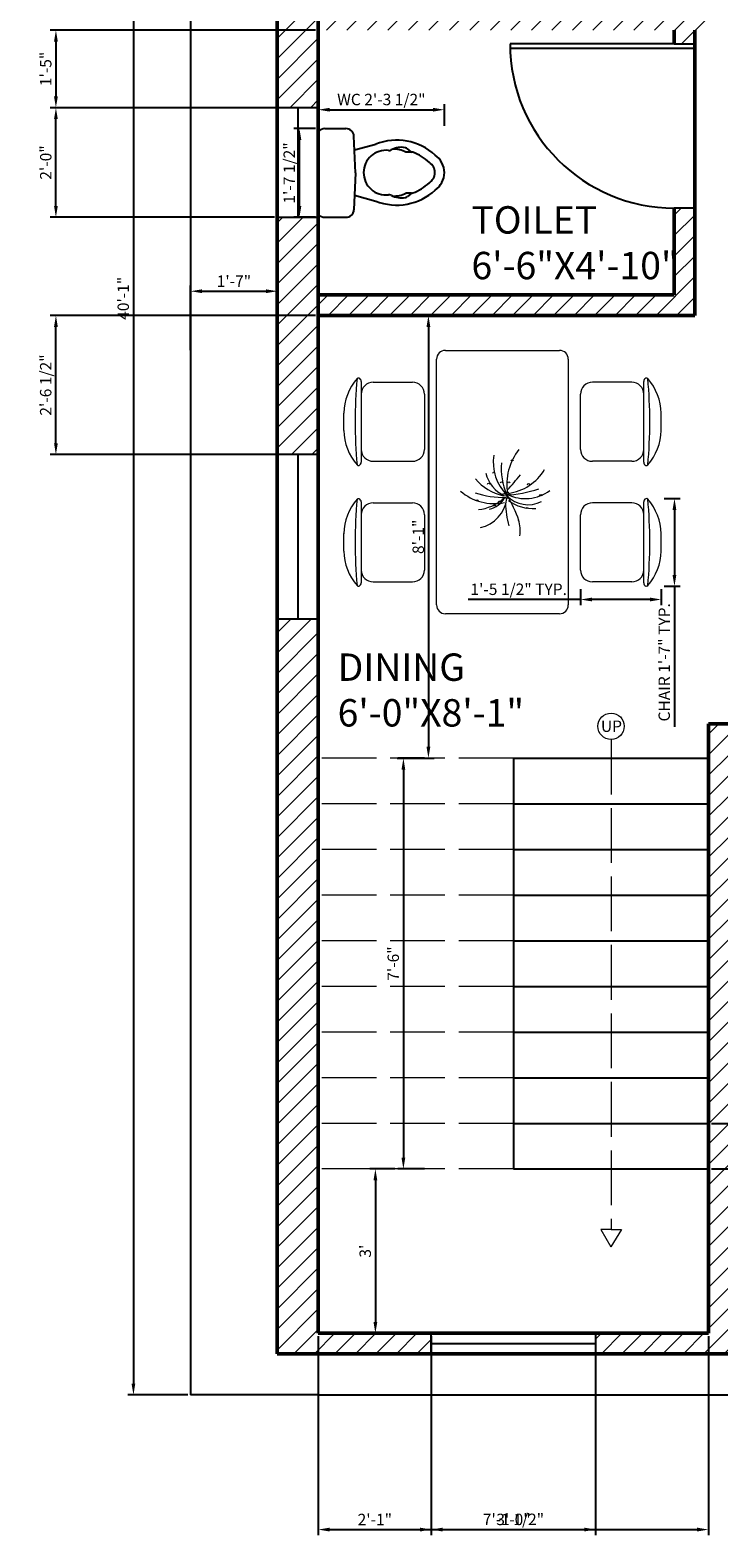
# Model space of a CAD drawing. Units: inches. Extents: x 3542 to 3908, y 2103 to 2666.
# Tile 1 of 4: x 3542 to 3693, y 2114 to 2444. Entities that reach past the tile are written whole.
import ezdxf

# ---------------------------------------------------------------- set-up
doc = ezdxf.new("R2010")
doc.units = ezdxf.units.IN
doc.linetypes.add('ACAD_ISO02W100', pattern=[15, 12, -3])
for name, color, linetype, lineweight in [('A-ANNO-DIMS', 2, 'Continuous', 18), ('A-ANNO-SYMB', 7, 'Continuous', 18), ('A-ANNO-TEXT', 7, 'Continuous', 25), ('A-AREA-IDEN', 7, 'Continuous', 25), ('A-DOOR', 3, 'Continuous', 25), ('A-FLOR-FIXT', 9, 'Continuous', 25), ('A-FLOR-STRS', 7, 'Continuous', 25), ('A-FLOR-STRS-OVHD', 7, 'ACAD_ISO02W100', 18), ('A-FLOR-STRS-PATH', 7, 'ACAD_ISO02W100', 18), ('A-FURN', 8, 'Continuous', 18), ('A-GLAZ', 5, 'Continuous', 25), ('A-WALL', 7, 'Continuous', 50), ('A-WALL-PATT', 252, 'Continuous', 13), ('C-PROP', 7, 'Continuous', 25)]:
    doc.layers.add(name, color=color, linetype=linetype, lineweight=lineweight)
doc.styles.get("Standard").update_dxf_attribs({"font": 'arial.ttf'})
doc.dimstyles.new('ISO-25', dxfattribs={"dimtxt": 2.5, "dimasz": 2.5, "dimexe": 1.25, "dimexo": 0.625, "dimtad": 1, "dimdec": 0, "dimlunit": 3, "dimtxsty": 'Standard', "dimcen": 2.5, "dimadec": 0, "dimazin": 0, "dimtfac": 1, "dimtdec": 0, "dimtmove": 0, "dimatfit": 3, "dimfxl": 1, "dimarcsym": 0})

# ---------------------------------------------------------------- blocks, each defined once
blk = doc.blocks.new('*D2')
at = {"layer": 'A-ANNO-DIMS', "color": 0, "lineweight": -2, "transparency": 16777216}
for p, q in [((3622.44, 2381.48), (3630.51, 2381.48)), ((3629.26, 2378.98), (3629.26, 2286.98)), ((3622.44, 2284.48), (3630.51, 2284.48))]:
    blk.add_line(p, q, dxfattribs=at)
at = {"layer": 'A-ANNO-DIMS', "color": 0, "transparency": 16777216}
for points in [[(3628.84, 2378.98), (3629.67, 2378.98), (3629.26, 2381.48)], [(3628.84, 2286.98), (3629.67, 2286.98), (3629.26, 2284.48)]]:
    blk.add_solid(points, dxfattribs=at)
at = {"layer": 'Defpoints', "color": 0, "transparency": 16777216}
for p in [(3621.81, 2381.48), (3621.81, 2284.48), (3629.26, 2284.48)]:
    blk.add_point(p, dxfattribs=at)
at = {"layer": 'A-ANNO-DIMS', "color": 0, "transparency": 16777216, "insert": (3627.36, 2332.98), "char_height": 2.5, "attachment_point": 5, "rotation": 90}
blk.add_mtext('8\'-1"', dxfattribs=at)
blk = doc.blocks.new('*D3')
at = {"layer": 'A-ANNO-DIMS', "color": 0, "lineweight": -2, "transparency": 16777216}
for p, q in [((3628.42, 2284.48), (3622.53, 2284.48)), ((3623.78, 2281.98), (3623.78, 2196.98)), ((3628.42, 2194.48), (3622.53, 2194.48))]:
    blk.add_line(p, q, dxfattribs=at)
at = {"layer": 'A-ANNO-DIMS', "color": 0, "transparency": 16777216}
for points in [[(3623.36, 2281.98), (3624.19, 2281.98), (3623.78, 2284.48)], [(3623.36, 2196.98), (3624.19, 2196.98), (3623.78, 2194.48)]]:
    blk.add_solid(points, dxfattribs=at)
at = {"layer": 'Defpoints', "color": 0, "transparency": 16777216}
for p in [(3629.05, 2284.48), (3623.78, 2194.48), (3629.05, 2194.48)]:
    blk.add_point(p, dxfattribs=at)
at = {"layer": 'A-ANNO-DIMS', "color": 0, "transparency": 16777216, "insert": (3621.88, 2239.48), "char_height": 2.5, "attachment_point": 5, "rotation": 90}
blk.add_mtext('7\'-6"', dxfattribs=at)
blk = doc.blocks.new('*D4')
at = {"layer": 'A-ANNO-DIMS', "color": 0, "lineweight": -2, "transparency": 16777216}
for p, q in [((3577.14, 2373.85), (3577.14, 2388.03)), ((3579.64, 2386.78), (3593.64, 2386.78)), ((3596.14, 2373.85), (3596.14, 2388.03))]:
    blk.add_line(p, q, dxfattribs=at)
at = {"layer": 'A-ANNO-DIMS', "color": 0, "transparency": 16777216}
for points in [[(3579.64, 2387.2), (3579.64, 2386.37), (3577.14, 2386.78)], [(3593.64, 2387.2), (3593.64, 2386.37), (3596.14, 2386.78)]]:
    blk.add_solid(points, dxfattribs=at)
at = {"layer": 'Defpoints', "color": 0, "transparency": 16777216}
for p in [(3596.14, 2386.78), (3577.14, 2373.23), (3596.14, 2373.23)]:
    blk.add_point(p, dxfattribs=at)
at = {"layer": 'A-ANNO-DIMS', "color": 0, "transparency": 16777216, "insert": (3586.64, 2388.66), "char_height": 2.5, "attachment_point": 5}
blk.add_mtext('1\'-7"', dxfattribs=at)
blk = doc.blocks.new('*D7')
at = {"layer": 'A-ANNO-DIMS', "color": 0, "lineweight": -2, "transparency": 16777216}
for p, q in [((3621.9, 2194.48), (3616.39, 2194.48)), ((3617.64, 2191.98), (3617.64, 2160.98)), ((3621.9, 2158.48), (3616.39, 2158.48))]:
    blk.add_line(p, q, dxfattribs=at)
at = {"layer": 'A-ANNO-DIMS', "color": 0, "transparency": 16777216}
for points in [[(3617.23, 2191.98), (3618.06, 2191.98), (3617.64, 2194.48)], [(3617.23, 2160.98), (3618.06, 2160.98), (3617.64, 2158.48)]]:
    blk.add_solid(points, dxfattribs=at)
at = {"layer": 'Defpoints', "color": 0, "transparency": 16777216}
for p in [(3622.53, 2194.48), (3617.64, 2158.48), (3622.53, 2158.48)]:
    blk.add_point(p, dxfattribs=at)
at = {"layer": 'A-ANNO-DIMS', "color": 0, "transparency": 16777216, "insert": (3615.74, 2176.48), "char_height": 2.5, "attachment_point": 5, "rotation": 90}
blk.add_mtext("3'", dxfattribs=at)
blk = doc.blocks.new('*D10')
at = {"layer": 'A-ANNO-DIMS', "color": 0, "lineweight": -2, "transparency": 16777216}
for p, q in [((3576.52, 2625.48), (3563.38, 2625.48)), ((3564.63, 2622.98), (3564.63, 2147.48)), ((3576.52, 2144.98), (3563.38, 2144.98))]:
    blk.add_line(p, q, dxfattribs=at)
at = {"layer": 'A-ANNO-DIMS', "color": 0, "transparency": 16777216}
for points in [[(3564.21, 2622.98), (3565.04, 2622.98), (3564.63, 2625.48)], [(3564.21, 2147.48), (3565.04, 2147.48), (3564.63, 2144.98)]]:
    blk.add_solid(points, dxfattribs=at)
at = {"layer": 'Defpoints', "color": 0, "transparency": 16777216}
for p in [(3577.14, 2625.48), (3564.63, 2144.98), (3577.14, 2144.98)]:
    blk.add_point(p, dxfattribs=at)
at = {"layer": 'A-ANNO-DIMS', "color": 0, "transparency": 16777216, "insert": (3562.72, 2385.23), "char_height": 2.5, "attachment_point": 5, "rotation": 90}
blk.add_mtext('40\'-1"', dxfattribs=at)
blk = doc.blocks.new('A$C1308471B')
at = {"ltscale": 20}
for p, q in [((0, 0.4607), (0, 0.0186)), ((0.0354, 0.4793), (0.1495, 0.4793)), ((0.2013, 0.2397), (0.1923, 0.4384)), ((0.1957, 0.3639), (0.3109, 0.3953)), ((0.5021, 0.3528), (0.4724, 0.3528)), ((0.4982, 0.3575), (0.4822, 0.3709)), ((0.2013, 0.2397), (0.1923, 0.0409)), ((0.1959, 0.1193), (0.3109, 0.0879)), ((0.5021, 0.1304), (0.4724, 0.1304)), ((0.4982, 0.1257), (0.4822, 0.1123)), ((0.0354, 0), (0.1495, 0))]:
    blk.add_line(p, q, dxfattribs=at)
for centre, radius, start, end in [((0.006, 0.4607), 0.006, 136.52689, 180), ((0.0354, 0.4328), 0.0465, 90, 136.52689), ((0.1495, 0.4365), 0.0429, 2.57554, 90), ((0.4248, 0.1104), 0.3068, 47.41345, 111.79241), ((0.3654, 0.2416), 0.1206, 83.35226, 180), ((0.3823, 0.3868), 0.0255, 263.35226, 298.57415), ((0.4494, 0.2636), 0.1148, 79.39683, 118.57415), ((0.405, 0.2159), 0.153, 63.50202, 90.45216), ((0.4658, 0.3513), 0.0255, 50, 79.39683), ((0.5146, 0.377), 0.0255, 230, 251.38812), ((0.5021, 0.3273), 0.0255, 70.3751, 90), ((0.4248, 0.1104), 0.2558, 46.61198, 70.3751), ((0.5654, 0.2416), 0.116, 0, 54.71147), ((0.5654, 0.2416), 0.065, 0, 57.29738), ((0.3654, 0.2416), 0.1206, 180, 276.64774), ((0.4248, 0.3728), 0.2558, 289.6249, 313.38802), ((0.5654, 0.2416), 0.065, 302.70262, 0), ((0.5654, 0.2416), 0.116, 305.28853, 0), ((0.4248, 0.3728), 0.3068, 248.20759, 312.58655), ((0.3823, 0.0964), 0.0255, 61.42585, 96.64774), ((0.4494, 0.2196), 0.1148, 241.42585, 280.60317), ((0.405, 0.2673), 0.153, 269.54784, 296.49798), ((0.4658, 0.1319), 0.0255, 280.60317, 310), ((0.5146, 0.1062), 0.0255, 108.61188, 130), ((0.5021, 0.1559), 0.0255, 270, 289.6249), ((0.006, 0.0186), 0.006, 180, 223.47311), ((0.0354, 0.0465), 0.0465, 223.47311, 270), ((0.1495, 0.0429), 0.0429, 270, 357.42446)]:
    blk.add_arc(centre, radius, start, end, dxfattribs=at)
blk = doc.blocks.new('DOOR-SWING-36IN')
for p, q in [((35, 0), (35, 40.5)), ((36, 4.5), (36, 40.5))]:
    blk.add_line(p, q)
blk.add_arc((36, 4.5), 36, 90, 180)
blk = doc.blocks.new('WIN-36IN')
for p, q in [((0, 36), (0, 0)), ((4.5, 36), (4.5, 0)), ((9, 0), (9, 36))]:
    blk.add_line(p, q)
blk = doc.blocks.new('CHAIR-DINING')
for p, q in [((3.85, 18.44), (3.85, 0.74)), ((6.45, 18.25), (15.1, 18.25)), ((17.7, 15.65), (17.7, 3.53)), ((0, 11.5), (0, 7.68)), ((6.45, 0.93), (15.1, 0.93))]:
    blk.add_line(p, q)
for centre, radius, start, end in [((12.14, 11.12), 12.14, 139.2735, 178.2349), ((106.89, 9.59), 104.38, 174.8023, 185.1977), ((3.23, 18.79), 0.385, 67.33, 139.2735), ((3.08, 18.44), 0.77, 0, 67.33), ((6.45, 15.65), 2.6, 90, 180), ((15.1, 15.65), 2.6, 0, 90), ((12.14, 8.06), 12.14, 181.7651, 220.7265), ((6.45, 3.53), 2.6, 180, 270), ((15.1, 3.53), 2.6, 270, 0), ((3.23, 0.38), 0.385, 220.7265, 292.67), ((3.08, 0.74), 0.77, 292.67, 0)]:
    blk.add_arc(centre, radius, start, end)
blk = doc.blocks.new('*D38')
at = {"layer": 'A-ANNO-DIMS', "color": 0, "lineweight": -2, "transparency": 16777216}
for p, q in [((3680.9, 2341.38), (3684.42, 2341.38)), ((3683.17, 2338.88), (3683.17, 2324.63)), ((3680.9, 2322.13), (3684.42, 2322.13)), ((3683.17, 2322.13), (3683.17, 2291.34))]:
    blk.add_line(p, q, dxfattribs=at)
at = {"layer": 'A-ANNO-DIMS', "color": 0, "transparency": 16777216}
for points in [[(3682.75, 2338.88), (3683.58, 2338.88), (3683.17, 2341.38)], [(3682.75, 2324.63), (3683.58, 2324.63), (3683.17, 2322.13)]]:
    blk.add_solid(points, dxfattribs=at)
at = {"layer": 'Defpoints', "color": 0, "transparency": 16777216}
for p in [(3680.28, 2341.38), (3680.28, 2322.13), (3683.17, 2322.13)]:
    blk.add_point(p, dxfattribs=at)
at = {"layer": 'A-ANNO-DIMS', "color": 0, "transparency": 16777216, "insert": (3681.25, 2305.48), "char_height": 2.5, "attachment_point": 5, "rotation": 90}
blk.add_mtext('CHAIR 1\'-7" TYP.', dxfattribs=at)
blk = doc.blocks.new('*D39')
at = {"layer": 'A-ANNO-DIMS', "color": 0, "lineweight": -2, "transparency": 16777216}
for p, q in [((3662.58, 2319.24), (3638, 2319.24)), ((3662.58, 2321.51), (3662.58, 2317.99)), ((3677.78, 2319.24), (3665.08, 2319.24)), ((3680.28, 2321.51), (3680.28, 2317.99))]:
    blk.add_line(p, q, dxfattribs=at)
at = {"layer": 'A-ANNO-DIMS', "color": 0, "transparency": 16777216}
for points in [[(3665.08, 2319.66), (3665.08, 2318.83), (3662.58, 2319.24)], [(3677.78, 2319.66), (3677.78, 2318.83), (3680.28, 2319.24)]]:
    blk.add_solid(points, dxfattribs=at)
at = {"layer": 'Defpoints', "color": 0, "transparency": 16777216}
for p in [(3662.58, 2322.13), (3680.28, 2322.13), (3662.58, 2319.24)]:
    blk.add_point(p, dxfattribs=at)
at = {"layer": 'A-ANNO-DIMS', "color": 0, "transparency": 16777216, "insert": (3649.04, 2321.16), "char_height": 2.5, "attachment_point": 5}
blk.add_mtext('1\'-5 1/2" TYP.', dxfattribs=at)
blk = doc.blocks.new('*D46')
at = {"layer": 'A-ANNO-DIMS', "color": 0, "lineweight": -2, "transparency": 16777216}
for p, q in [((3605.14, 2423.03), (3605.14, 2427.79)), ((3632.75, 2423.03), (3632.75, 2427.79)), ((3607.64, 2426.54), (3630.25, 2426.54))]:
    blk.add_line(p, q, dxfattribs=at)
at = {"layer": 'A-ANNO-DIMS', "color": 0, "transparency": 16777216}
for points in [[(3607.64, 2426.96), (3607.64, 2426.13), (3605.14, 2426.54)], [(3630.25, 2426.96), (3630.25, 2426.13), (3632.75, 2426.54)]]:
    blk.add_solid(points, dxfattribs=at)
at = {"layer": 'Defpoints', "color": 0, "transparency": 16777216}
for p in [(3632.75, 2426.54), (3605.14, 2422.4), (3632.75, 2422.4)]:
    blk.add_point(p, dxfattribs=at)
at = {"layer": 'A-ANNO-DIMS', "color": 0, "transparency": 16777216, "insert": (3618.95, 2428.46), "char_height": 2.5, "attachment_point": 5}
blk.add_mtext('WC 2\'-3 1/2"', dxfattribs=at)
blk = doc.blocks.new('*D47')
at = {"layer": 'A-ANNO-DIMS', "color": 0, "lineweight": -2, "transparency": 16777216}
for p, q in [((3604.52, 2422.4), (3599.75, 2422.4)), ((3601, 2405.48), (3601, 2419.9)), ((3604.52, 2402.98), (3599.75, 2402.98))]:
    blk.add_line(p, q, dxfattribs=at)
at = {"layer": 'A-ANNO-DIMS', "color": 0, "transparency": 16777216}
for points in [[(3600.59, 2419.9), (3601.42, 2419.9), (3601, 2422.4)], [(3600.59, 2405.48), (3601.42, 2405.48), (3601, 2402.98)]]:
    blk.add_solid(points, dxfattribs=at)
at = {"layer": 'Defpoints', "color": 0, "transparency": 16777216}
for p in [(3601, 2422.4), (3605.14, 2422.4), (3605.14, 2402.98)]:
    blk.add_point(p, dxfattribs=at)
at = {"layer": 'A-ANNO-DIMS', "color": 0, "transparency": 16777216, "insert": (3599.09, 2412.69), "char_height": 2.5, "attachment_point": 5, "rotation": 90}
blk.add_mtext('1\'-7 1/2"', dxfattribs=at)
blk = doc.blocks.new('*D48')
at = {"layer": 'A-ANNO-DIMS', "color": 0, "lineweight": -2, "transparency": 16777216}
for p, q in [((3605.14, 2157.85), (3605.14, 2114.23)), ((3690.64, 2157.85), (3690.64, 2114.23)), ((3607.64, 2115.48), (3688.14, 2115.48))]:
    blk.add_line(p, q, dxfattribs=at)
at = {"layer": 'A-ANNO-DIMS', "color": 0, "transparency": 16777216}
for points in [[(3607.64, 2115.9), (3607.64, 2115.06), (3605.14, 2115.48)], [(3688.14, 2115.9), (3688.14, 2115.06), (3690.64, 2115.48)]]:
    blk.add_solid(points, dxfattribs=at)
at = {"layer": 'Defpoints', "color": 0, "transparency": 16777216}
for p in [(3605.14, 2158.48), (3690.64, 2158.48), (3690.64, 2115.48)]:
    blk.add_point(p, dxfattribs=at)
at = {"layer": 'A-ANNO-DIMS', "color": 0, "transparency": 16777216, "insert": (3647.89, 2117.4), "char_height": 2.5, "attachment_point": 5}
blk.add_mtext('7\'-1 1/2"', dxfattribs=at)
blk = doc.blocks.new('*D49')
at = {"layer": 'A-ANNO-DIMS', "color": 0, "lineweight": -2, "transparency": 16777216}
for p, q in [((3691.27, 2204.48), (3907.39, 2204.48)), ((3906.14, 2196.98), (3906.14, 2201.98)), ((3691.27, 2194.48), (3907.39, 2194.48))]:
    blk.add_line(p, q, dxfattribs=at)
at = {"layer": 'A-ANNO-DIMS', "color": 0, "transparency": 16777216}
for points in [[(3905.73, 2201.98), (3906.56, 2201.98), (3906.14, 2204.48)], [(3905.73, 2196.98), (3906.56, 2196.98), (3906.14, 2194.48)]]:
    blk.add_solid(points, dxfattribs=at)
at = {"layer": 'Defpoints', "color": 0, "transparency": 16777216}
for p in [(3690.64, 2204.48), (3906.14, 2204.48), (3690.64, 2194.48)]:
    blk.add_point(p, dxfattribs=at)
at = {"layer": 'A-ANNO-DIMS', "color": 0, "transparency": 16777216, "insert": (3904.24, 2199.48), "char_height": 2.5, "attachment_point": 5, "rotation": 90}
blk.add_mtext('0\'-10"', dxfattribs=at)
blk = doc.blocks.new('*D54')
at = {"layer": 'A-ANNO-DIMS', "color": 0, "lineweight": -2, "transparency": 16777216}
for p, q in [((3595.52, 2426.98), (3546.39, 2426.98)), ((3547.64, 2405.48), (3547.64, 2424.48)), ((3595.52, 2402.98), (3546.39, 2402.98))]:
    blk.add_line(p, q, dxfattribs=at)
at = {"layer": 'A-ANNO-DIMS', "color": 0, "transparency": 16777216}
for points in [[(3547.23, 2424.48), (3548.06, 2424.48), (3547.64, 2426.98)], [(3547.23, 2405.48), (3548.06, 2405.48), (3547.64, 2402.98)]]:
    blk.add_solid(points, dxfattribs=at)
at = {"layer": 'Defpoints', "color": 0, "transparency": 16777216}
for p in [(3547.64, 2426.98), (3596.14, 2426.98), (3596.14, 2402.98)]:
    blk.add_point(p, dxfattribs=at)
at = {"layer": 'A-ANNO-DIMS', "color": 0, "transparency": 16777216, "insert": (3545.74, 2414.98), "char_height": 2.5, "attachment_point": 5, "rotation": 90}
blk.add_mtext('2\'-0"', dxfattribs=at)
blk = doc.blocks.new('*D55')
at = {"layer": 'A-ANNO-DIMS', "color": 0, "lineweight": -2, "transparency": 16777216}
for p, q in [((3604.52, 2443.98), (3546.39, 2443.98)), ((3547.64, 2441.48), (3547.64, 2429.48)), ((3604.52, 2426.98), (3546.39, 2426.98))]:
    blk.add_line(p, q, dxfattribs=at)
at = {"layer": 'A-ANNO-DIMS', "color": 0, "transparency": 16777216}
for points in [[(3547.23, 2441.48), (3548.06, 2441.48), (3547.64, 2443.98)], [(3547.23, 2429.48), (3548.06, 2429.48), (3547.64, 2426.98)]]:
    blk.add_solid(points, dxfattribs=at)
at = {"layer": 'Defpoints', "color": 0, "transparency": 16777216}
for p in [(3605.14, 2443.98), (3547.64, 2426.98), (3605.14, 2426.98)]:
    blk.add_point(p, dxfattribs=at)
at = {"layer": 'A-ANNO-DIMS', "color": 0, "transparency": 16777216, "insert": (3545.74, 2435.48), "char_height": 2.5, "attachment_point": 5, "rotation": 90}
blk.add_mtext('1\'-5"', dxfattribs=at)
blk = doc.blocks.new('*D58')
at = {"layer": 'A-ANNO-DIMS', "color": 0, "lineweight": -2, "transparency": 16777216}
for p, q in [((3629.89, 2157.85), (3629.89, 2114.23)), ((3665.89, 2157.85), (3665.89, 2114.23)), ((3632.39, 2115.48), (3663.39, 2115.48))]:
    blk.add_line(p, q, dxfattribs=at)
at = {"layer": 'A-ANNO-DIMS', "color": 0, "transparency": 16777216}
for points in [[(3632.39, 2115.9), (3632.39, 2115.06), (3629.89, 2115.48)], [(3663.39, 2115.9), (3663.39, 2115.06), (3665.89, 2115.48)]]:
    blk.add_solid(points, dxfattribs=at)
at = {"layer": 'Defpoints', "color": 0, "transparency": 16777216}
for p in [(3629.89, 2158.48), (3665.89, 2158.48), (3665.89, 2115.48)]:
    blk.add_point(p, dxfattribs=at)
at = {"layer": 'A-ANNO-DIMS', "color": 0, "transparency": 16777216, "insert": (3647.89, 2117.38), "char_height": 2.5, "attachment_point": 5}
blk.add_mtext('3\'-0"', dxfattribs=at)
blk = doc.blocks.new('*D59')
at = {"layer": 'A-ANNO-DIMS', "color": 0, "lineweight": -2, "transparency": 16777216}
for p, q in [((3605.14, 2157.85), (3605.14, 2114.23)), ((3629.89, 2157.85), (3629.89, 2114.23)), ((3607.64, 2115.48), (3627.39, 2115.48))]:
    blk.add_line(p, q, dxfattribs=at)
at = {"layer": 'A-ANNO-DIMS', "color": 0, "transparency": 16777216}
for points in [[(3607.64, 2115.9), (3607.64, 2115.06), (3605.14, 2115.48)], [(3627.39, 2115.9), (3627.39, 2115.06), (3629.89, 2115.48)]]:
    blk.add_solid(points, dxfattribs=at)
at = {"layer": 'Defpoints', "color": 0, "transparency": 16777216}
for p in [(3605.14, 2158.48), (3629.89, 2158.48), (3629.89, 2115.48)]:
    blk.add_point(p, dxfattribs=at)
at = {"layer": 'A-ANNO-DIMS', "color": 0, "transparency": 16777216, "insert": (3617.52, 2117.36), "char_height": 2.5, "attachment_point": 5}
blk.add_mtext('2\'-1"', dxfattribs=at)
blk = doc.blocks.new('*D61')
at = {"layer": 'A-ANNO-DIMS', "color": 0, "lineweight": -2, "transparency": 16777216}
for p, q in [((3604.52, 2381.48), (3546.39, 2381.48)), ((3547.64, 2353.48), (3547.64, 2378.98)), ((3604.52, 2350.98), (3546.39, 2350.98))]:
    blk.add_line(p, q, dxfattribs=at)
at = {"layer": 'A-ANNO-DIMS', "color": 0, "transparency": 16777216}
for points in [[(3547.23, 2378.98), (3548.06, 2378.98), (3547.64, 2381.48)], [(3547.23, 2353.48), (3548.06, 2353.48), (3547.64, 2350.98)]]:
    blk.add_solid(points, dxfattribs=at)
at = {"layer": 'Defpoints', "color": 0, "transparency": 16777216}
for p in [(3547.64, 2381.48), (3605.14, 2381.48), (3605.14, 2350.98)]:
    blk.add_point(p, dxfattribs=at)
at = {"layer": 'A-ANNO-DIMS', "color": 0, "transparency": 16777216, "insert": (3545.73, 2366.23), "char_height": 2.5, "attachment_point": 5, "rotation": 90}
blk.add_mtext('2\'-6 1/2"', dxfattribs=at)

msp = doc.modelspace()

# ---------------------------------------------------------------- hatches: boundary and pattern name
at = {"layer": 'A-WALL-PATT'}
h = msp.add_hatch(dxfattribs=at)
h.set_pattern_fill('ANSI31', color=256)
h.paths.add_polyline_path([(3864.64, 2601.48), (3596.14, 2601.48), (3596.14, 2550.48), (3605.14, 2550.48), (3605.14, 2592.48), (3855.64, 2592.48), (3855.64, 2550.48), (3864.64, 2550.48)])
h.paths.add_polyline_path([(3735.64, 2592.48), (3731.14, 2592.48), (3731.14, 2448.48), (3728.14, 2448.48), (3728.14, 2443.98), (3738.64, 2443.98), (3738.64, 2448.48), (3735.64, 2448.48)])
h.paths.add_polyline_path([(3855.64, 2448.48), (3774.64, 2448.48), (3774.64, 2443.98), (3855.64, 2443.98)])
h.paths.add_polyline_path([(3605.14, 2490.48), (3596.14, 2490.48), (3596.14, 2426.98), (3605.14, 2426.98)])
h.paths.add_polyline_path([(3605.14, 2402.98), (3596.14, 2402.98), (3596.14, 2350.98), (3605.14, 2350.98)])
h.paths.add_polyline_path([(3692.14, 2448.48), (3605.14, 2448.48), (3605.14, 2443.98), (3683.14, 2443.98), (3683.14, 2440.98), (3687.64, 2440.98), (3687.64, 2443.98), (3692.14, 2443.98)])
h.paths.add_polyline_path([(3687.64, 2404.98), (3683.14, 2404.98), (3683.14, 2385.98), (3605.14, 2385.98), (3605.14, 2381.48), (3687.64, 2381.48)])
h.paths.add_polyline_path([(3864.64, 2490.48), (3855.64, 2490.48), (3855.64, 2397.98), (3864.64, 2397.98)])
h.paths.add_polyline_path([(3864.64, 2337.98), (3855.64, 2337.98), (3855.64, 2269.48), (3864.64, 2269.48)])
h.paths.add_polyline_path([(3864.64, 2233.48), (3855.64, 2233.48), (3855.64, 2215.48), (3831.64, 2215.48), (3831.64, 2206.48), (3864.64, 2206.48)])
h.paths.add_polyline_path([(3771.64, 2215.48), (3740.31, 2215.48), (3740.31, 2206.48), (3771.64, 2206.48)])
h.paths.add_polyline_path([(3747.64, 2287.48), (3750.64, 2287.48), (3750.64, 2291.98), (3743.14, 2291.98), (3743.14, 2215.48), (3747.64, 2215.48)])
h.paths.add_polyline_path([(3706.76, 2215.48), (3695.14, 2215.48), (3695.14, 2291.98), (3690.64, 2291.98), (3690.64, 2206.48), (3690.64, 2158.48), (3665.89, 2158.48), (3665.89, 2153.98), (3690.64, 2153.98), (3699.64, 2153.98), (3699.64, 2206.48), (3706.76, 2206.48)])
h.paths.add_polyline_path([(3605.14, 2314.98), (3596.14, 2314.98), (3596.14, 2153.98), (3629.89, 2153.98), (3629.89, 2158.48), (3605.14, 2158.48)])

# ---------------------------------------------------------------- linework, layer by layer
at = {"layer": 'A-ANNO-SYMB'}
for p, q in [((3669.27, 2181.21), (3667.01, 2181.22)), ((3667.01, 2181.22), (3669.26, 2177.43)), ((3671.53, 2181.21), (3669.26, 2177.43)), ((3669.27, 2181.21), (3671.53, 2181.21))]:
    msp.add_line(p, q, dxfattribs=at)
msp.add_circle((3669.27, 2291.46), 2.89, dxfattribs=at)
at = {"layer": 'A-DOOR'}
for p, q in [((3683.14, 2440.98), (3687.64, 2440.98)), ((3687.64, 2404.98), (3683.14, 2404.98))]:
    msp.add_line(p, q, dxfattribs=at)
at = {"layer": 'A-FLOR-STRS'}
for p, q in [((3647.89, 2284.48), (3690.64, 2284.48)), ((3647.89, 2284.48), (3647.89, 2194.48)), ((3647.89, 2274.48), (3690.64, 2274.48)), ((3647.89, 2264.48), (3690.64, 2264.48)), ((3647.89, 2254.48), (3690.64, 2254.48)), ((3647.89, 2244.48), (3690.64, 2244.48)), ((3647.89, 2234.48), (3690.64, 2234.48)), ((3647.89, 2224.48), (3690.64, 2224.48)), ((3647.89, 2214.48), (3690.64, 2214.48)), ((3647.89, 2204.48), (3690.64, 2204.48)), ((3647.89, 2194.48), (3690.64, 2194.48))]:
    msp.add_line(p, q, dxfattribs=at)
at = {"layer": 'A-FLOR-STRS-OVHD'}
for p, q in [((3647.89, 2284.48), (3605.14, 2284.48)), ((3647.89, 2274.48), (3605.14, 2274.48)), ((3647.89, 2264.48), (3605.14, 2264.48)), ((3647.89, 2254.48), (3605.14, 2254.48)), ((3647.89, 2244.48), (3605.14, 2244.48)), ((3647.89, 2234.48), (3605.14, 2234.48)), ((3647.89, 2224.48), (3605.14, 2224.48)), ((3647.89, 2214.48), (3605.14, 2214.48)), ((3647.89, 2204.48), (3605.14, 2204.48)), ((3647.89, 2194.48), (3605.14, 2194.48))]:
    msp.add_line(p, q, dxfattribs=at)
at = {"layer": 'A-FLOR-STRS-PATH'}
msp.add_line((3669.27, 2288.56), (3669.27, 2181.21), dxfattribs=at)
at = {"layer": 'A-FURN'}
for p, q in [((3631.05, 2318.04), (3631.05, 2371.91)), ((3632.98, 2373.83), (3657.99, 2373.83)), ((3659.91, 2371.91), (3659.91, 2318.04)), ((3657.99, 2316.11), (3632.98, 2316.11))]:
    msp.add_line(p, q, dxfattribs=at)
for points in [[(3647.39, 2349.6, -1), (3647.85, 2349.6, -1)], [(3643.37, 2346.94, -1), (3643.83, 2346.94, -1)], [(3642.21, 2344.53, -1), (3642.67, 2344.53, -1)], [(3645.06, 2344.78, -1), (3645.52, 2344.78, -1)], [(3645.59, 2342.24, -1), (3646.05, 2342.24, -1)], [(3646.23, 2341.86, -1), (3646.69, 2341.86, -1)], [(3646.33, 2342.62, -1), (3646.79, 2342.62, -1)], [(3646.65, 2344.78, -1), (3647.11, 2344.78, -1)], [(3646.75, 2342.11, -1), (3647.22, 2342.11, -1)], [(3650.99, 2344.4, -1), (3651.45, 2344.4, -1)], [(3653.63, 2341.99, -1), (3654.09, 2341.99, -1)], [(3639.67, 2340.85, -1), (3640.13, 2340.85, -1)], [(3643.58, 2339.7, -1), (3644.04, 2339.7, -1)], [(3644.64, 2340.59, -1), (3645.1, 2340.59, -1)], [(3646.01, 2341.35, -1), (3646.48, 2341.35, -1)], [(3650.67, 2339.19, -1), (3651.13, 2339.19, -1)]]:
    msp.add_lwpolyline(points, format="xyb", dxfattribs=at)
for centre, radius, start, end in [((3632.98, 2371.91), 1.92, 90, 180), ((3657.99, 2371.91), 1.92, 0, 90), ((3658.93, 2344.4), 12.51, 141.7667, 188.7504), ((3653.46, 2349.25), 9.99, 170.6238, 225.5139), ((3658.52, 2347.84), 13.3, 174.0363, 204.9112), ((3648.14, 2352.91), 11.21, 220.2234, 256.9548), ((3648.92, 2348.67), 7.32, 193.7047, 245.9044), ((3595.93, 2389.95), 68.88, 317.3201, 320.9512), ((3645.26, 2353.45), 11.06, 277.8622, 328.685), ((3643.69, 2351.51), 11.27, 229.0185, 281.4484), ((3645.68, 2360.93), 19.33, 251.271, 271.6714), ((3645.2, 2366.81), 24.71, 272.1756, 289.4751), ((3619.73, 2326.05), 31.18, 19.639, 31.0127), ((3651.12, 2346.51), 6.5, 224.0898, 297.0091), ((3650.48, 2350.37), 9.02, 244.2367, 306.6769), ((3639.15, 2348.84), 9.96, 276.1376, 311.2419), ((3639.1, 2342.26), 7.41, 281.9716, 353.0096), ((3641.68, 2343.83), 4.86, 281.5421, 331.1099), ((3664.99, 2340.63), 18.85, 180.8895, 196.1439), ((3652.16, 2348.13), 8.96, 233.0442, 274.1259), ((3640.93, 2334.18), 8.44, 353.5186, 17.0544), ((3632.98, 2318.04), 1.92, 180, 270), ((3657.99, 2318.04), 1.92, 270, 0)]:
    msp.add_arc(centre, radius, start, end, dxfattribs=at)
at = {"layer": 'A-GLAZ'}
for p, q in [((3596.14, 2426.98), (3596.14, 2402.98)), ((3605.14, 2426.98), (3596.14, 2426.98)), ((3600.64, 2426.98), (3600.64, 2402.98)), ((3605.14, 2402.98), (3605.14, 2426.98)), ((3596.14, 2402.98), (3605.14, 2402.98)), ((3605.14, 2350.98), (3596.14, 2350.98)), ((3596.14, 2314.98), (3605.14, 2314.98)), ((3629.89, 2158.48), (3665.89, 2158.48)), ((3629.89, 2153.98), (3629.89, 2158.48)), ((3665.89, 2158.48), (3665.89, 2153.98)), ((3629.89, 2156.23), (3665.89, 2156.23)), ((3665.89, 2153.98), (3629.89, 2153.98))]:
    msp.add_line(p, q, dxfattribs=at)
at = {"layer": 'A-WALL'}
for p, q in [((3596.14, 2601.48), (3596.14, 2153.98)), ((3605.14, 2592.48), (3605.14, 2158.48)), ((3683.14, 2443.98), (3683.14, 2440.98)), ((3687.64, 2443.98), (3687.64, 2381.48)), ((3683.14, 2404.98), (3683.14, 2385.98)), ((3605.14, 2385.98), (3683.14, 2385.98)), ((3605.14, 2381.48), (3687.64, 2381.48)), ((3690.64, 2291.98), (3690.64, 2206.48)), ((3690.64, 2291.98), (3695.14, 2291.98)), ((3690.64, 2206.48), (3690.64, 2158.48)), ((3605.14, 2158.48), (3690.64, 2158.48)), ((3596.14, 2153.98), (3690.64, 2153.98)), ((3690.64, 2153.98), (3699.64, 2153.98))]:
    msp.add_line(p, q, dxfattribs=at)
at = {"layer": 'C-PROP'}
for p, q in [((3577.14, 2601.48), (3577.14, 2144.98)), ((3596.14, 2144.98), (3577.14, 2144.98)), ((3605.14, 2144.98), (3596.14, 2144.98)), ((3605.14, 2144.98), (3690.64, 2144.98)), ((3690.64, 2144.98), (3864.64, 2144.98))]:
    msp.add_line(p, q, dxfattribs=at)

# ---------------------------------------------------------------- block references
at = {"layer": 'A-DOOR', "rotation": 90.00000000000033}
msp.add_blockref('DOOR-SWING-36IN', (3687.64, 2404.98), dxfattribs=at)
at = {"layer": 'A-FLOR-FIXT', "xscale": 40.51907366769409, "yscale": 40.51907366769409, "zscale": 40.51907366769409}
msp.add_blockref('A$C1308471B', (3605.14, 2402.98), dxfattribs=at)
at = {"layer": 'A-FURN'}
for p in [(3610.69, 2348.6), (3610.69, 2322.17)]:
    msp.add_blockref('CHAIR-DINING', p, dxfattribs=at)
at = {"layer": 'A-FURN', "rotation": 180}
for p in [(3680.28, 2367.77), (3680.28, 2341.35)]:
    msp.add_blockref('CHAIR-DINING', p, dxfattribs=at)
at = {"layer": 'A-GLAZ'}
msp.add_blockref('WIN-36IN', (3596.14, 2314.98), dxfattribs=at)

# ---------------------------------------------------------------- texts
at = {"layer": 'A-ANNO-TEXT', "insert": (3667.06, 2292.73), "char_height": 2.5, "attachment_point": 1}
msp.add_mtext('UP', dxfattribs=at)
at = {"layer": 'A-AREA-IDEN', "char_height": 6, "attachment_point": 1}
for s, insert in [('TOILET\\P6\'-6"X4\'-10"', (3638.69, 2405.41)), ('DINING\\P6\'-0"X8\'-1"', (3609.37, 2307.42))]:
    msp.add_mtext(s, dxfattribs=dict(at, insert=insert))

# ---------------------------------------------------------------- dimensions: what is measured, and where the dimension line sits
at = {"layer": 'A-ANNO-DIMS'}
for base, p1, p2, override, picture, middle in [((3564.62592245, 2144.97915136), (3577.14448065, 2625.47915136), (3577.14448065, 2144.97915136), {"dimclrd": 0, "dimclre": 0, "dimclrt": 0}, '*D10', (3562.72448998, 2385.22915136)), ((3547.64, 2426.98), (3605.14, 2443.98), (3605.14, 2426.98), {"dimdec": 1, "dimlfac": 1, "dimrnd": 0, "dimzin": 1, "dimdsep": 46, "dimlunit": 4, "dimfrac": 2}, '*D55', (3545.74, 2435.48)), ((3547.64, 2426.98), (3596.14, 2402.98), (3596.14, 2426.98), {"dimdec": 1, "dimlfac": 1, "dimrnd": 0, "dimzin": 1, "dimdsep": 46, "dimlunit": 4, "dimfrac": 2}, '*D54', (3545.74, 2414.98)), ((3601, 2422.4), (3605.14, 2402.98), (3605.14, 2422.4), {"dimdec": 1, "dimlfac": 1, "dimrnd": 0, "dimzin": 1, "dimdsep": 46, "dimlunit": 4, "dimfrac": 2}, '*D47', (3599.09, 2412.69)), ((3547.64, 2381.48), (3605.14, 2350.98), (3605.14, 2381.48), {"dimdec": 1, "dimlfac": 1, "dimrnd": 0, "dimzin": 1, "dimdsep": 46, "dimlunit": 4, "dimfrac": 2}, '*D61', (3545.73, 2366.23)), ((3629.26, 2284.48), (3621.81, 2381.48), (3621.81, 2284.48), {"dimclrd": 0, "dimclre": 0, "dimclrt": 0}, '*D2', (3627.36, 2332.98)), ((3623.78, 2194.48), (3629.05, 2284.48), (3629.05, 2194.48), {"dimclrd": 0, "dimclre": 0, "dimclrt": 0}, '*D3', (3621.88, 2239.48)), ((3906.14, 2204.48), (3690.64, 2194.48), (3690.64, 2204.48), {"dimdec": 1, "dimlfac": 1, "dimrnd": 0, "dimzin": 1, "dimdsep": 46, "dimlunit": 4, "dimfrac": 2}, '*D49', (3904.24, 2199.48)), ((3617.64, 2158.48), (3622.53, 2194.48), (3622.53, 2158.48), {"dimclrd": 0, "dimclre": 0, "dimclrt": 0}, '*D7', (3615.74, 2176.48))]:
    dim = msp.add_linear_dim(base=base, p1=p1, p2=p2, angle=90, dimstyle='ISO-25', override=override, dxfattribs=at)
    dim.commit()
    dim.dimension.update_dxf_attribs({"geometry": picture, "text_midpoint": middle})
dim = msp.add_linear_dim(base=(3632.75, 2426.54), p1=(3605.14, 2422.4), p2=(3632.75, 2422.4), text='WC <>', dimstyle='ISO-25', override={"dimdec": 1, "dimlfac": 1, "dimrnd": 0, "dimzin": 1, "dimdsep": 46, "dimlunit": 4, "dimfrac": 2}, dxfattribs=at)
dim.commit()
dim.dimension.update_dxf_attribs({"geometry": '*D46', "text_midpoint": (3618.95, 2428.46)})
for base, p1, p2, override, picture, middle in [((3596.14, 2386.78), (3577.14, 2373.23), (3596.14, 2373.23), {"dimclrd": 0, "dimclre": 0, "dimclrt": 0}, '*D4', (3586.64, 2388.66)), ((3690.64, 2115.48), (3605.14, 2158.48), (3690.64, 2158.48), {"dimdec": 1, "dimlfac": 1, "dimrnd": 0, "dimzin": 1, "dimdsep": 46, "dimlunit": 4, "dimfrac": 2}, '*D48', (3647.89, 2117.4)), ((3629.894481, 2115.479151), (3605.144481, 2158.479151), (3629.894481, 2158.479151), {"dimdec": 1, "dimlfac": 1, "dimrnd": 0, "dimzin": 1, "dimdsep": 46, "dimlunit": 4, "dimfrac": 2}, '*D59', (3617.519481, 2117.35926696)), ((3665.89, 2115.48), (3629.89, 2158.48), (3665.89, 2158.48), {"dimdec": 1, "dimlfac": 1, "dimrnd": 0, "dimzin": 1, "dimdsep": 46, "dimlunit": 4, "dimfrac": 2}, '*D58', (3647.89, 2117.38))]:
    dim = msp.add_linear_dim(base=base, p1=p1, p2=p2, dimstyle='ISO-25', override=override, dxfattribs=at)
    dim.commit()
    dim.dimension.update_dxf_attribs({"geometry": picture, "text_midpoint": middle})
for base, p1, p2, angle, text, picture, middle in [((3683.1668, 2322.1322), (3680.2794, 2341.3814), (3680.2794, 2322.1322), 270, 'CHAIR <> TYP.', '*D38', (3681.2492, 2305.484)), ((3662.58, 2319.24), (3680.28, 2322.13), (3662.58, 2322.13), 180, '<> TYP.', '*D39', (3649.04, 2321.16))]:
    dim = msp.add_linear_dim(base=base, p1=p1, p2=p2, angle=angle, text=text, dimstyle='ISO-25', override={"dimdec": 1, "dimlfac": 1, "dimrnd": 0, "dimzin": 1, "dimdsep": 46, "dimlunit": 4, "dimfrac": 2}, dxfattribs=at)
    dim.commit()
    dim.dimension.update_dxf_attribs({"geometry": picture, "text_midpoint": middle})

doc.saveas('drawing.dxf')
